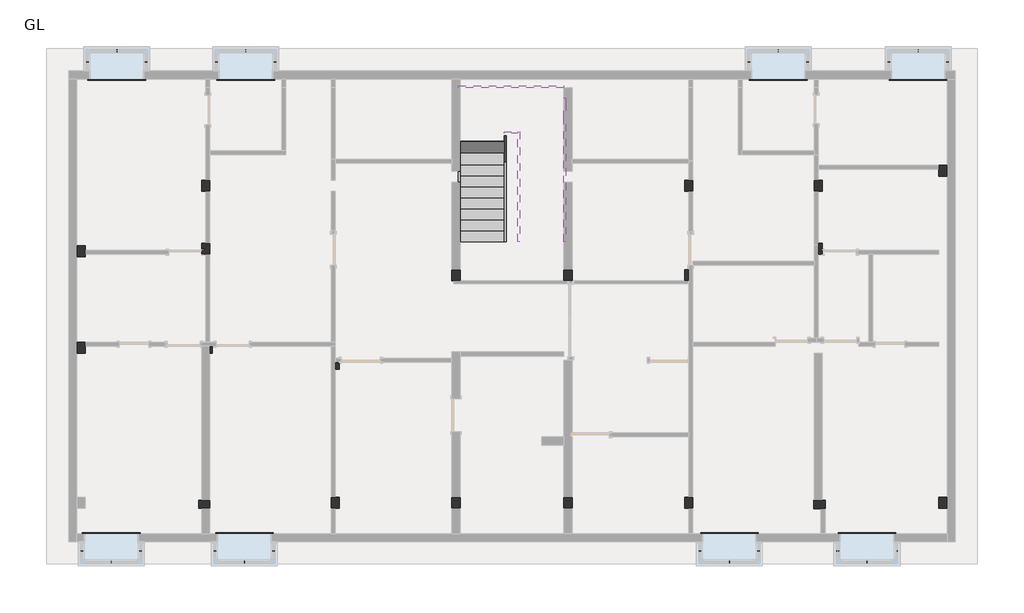
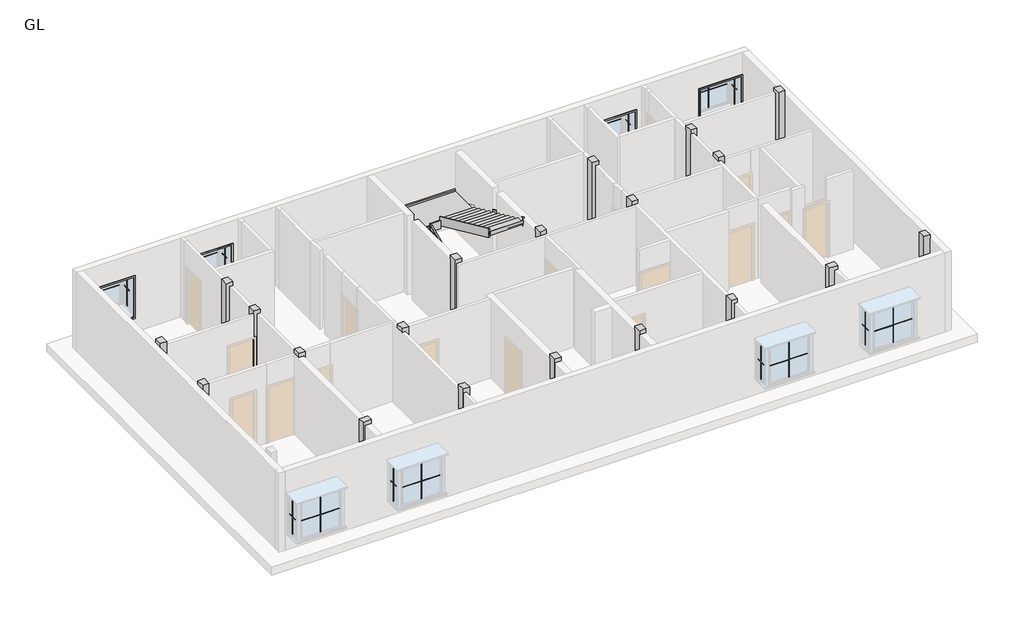
# One storey, part 3 of 3: 32 proxies, 20 columns, 6 members, 1 stair flight.
"""IFC4 building model written with IfcOpenShell, lengths in millimetres."""

from ifc_helpers import new_model, si_unit, frame, origin, place, context, project, spatial, polyline, outline, extrude, faceted_brep, transform, mapped, element, save
from components import m_muntin_pattern_2x2_m_muntin_pattern_2x2_c1fd4460, m_muntin_pattern_2x2_m_muntin_pattern_2x2_777b163a, m_trim_window_interior_flat_picture_frame_44e8afef, stair_flight_f8c5991c

model = new_model("IFC4")

# Units and contexts
model_context = context("Model", 3, world=origin())
ifc_project = project(units=[si_unit("LENGTHUNIT", "METRE", prefix="MILLI")], contexts=[model_context])

# Site, building, storey
site = spatial("IfcSite", under=ifc_project)
building = spatial("IfcBuilding", under=site)
storey = spatial("IfcBuildingStorey", under=building, Name="GL", Elevation=3200.4)

# Proxies
placement = place(None, origin())
m_muntin_pattern_2x2_m_muntin_pattern_2x2_shape = m_muntin_pattern_2x2_m_muntin_pattern_2x2_c1fd4460(model_context)
element("IfcBuildingElementProxy", 1, Name="M_Muntin Pattern_2x2 : M_Muntin Pattern_2x2", ObjectType="M_Muntin Pattern_2x2 : M_Muntin Pattern_2x2", at=placement, inside=storey, context=model_context, shape_type="MappedRepresentation", body=[
    mapped(m_muntin_pattern_2x2_m_muntin_pattern_2x2_shape, transform((-11500.7987957, -5499.9182661, 3921.05), x_axis=(-1.0, 0.0, 0.0), y_axis=(0.0, -1.0, 0.0), z_axis=(0.0, 0.0, 1.0))),
])
element("IfcBuildingElementProxy", 2, Name="M_Muntin Pattern_2x2 : M_Muntin Pattern_2x2", ObjectType="M_Muntin Pattern_2x2 : M_Muntin Pattern_2x2", at=placement, inside=storey, context=model_context, shape_type="MappedRepresentation", body=[
    mapped(m_muntin_pattern_2x2_m_muntin_pattern_2x2_shape, transform((-7819.250543, -5499.9182661, 3921.05), x_axis=(-1.0, 0.0, 0.0), y_axis=(0.0, -1.0, 0.0), z_axis=(0.0, 0.0, 1.0))),
])
element("IfcBuildingElementProxy", 3, Name="M_Muntin Pattern_2x2 : M_Muntin Pattern_2x2", ObjectType="M_Muntin Pattern_2x2 : M_Muntin Pattern_2x2", at=placement, inside=storey, context=model_context, shape_type="MappedRepresentation", body=[
    mapped(m_muntin_pattern_2x2_m_muntin_pattern_2x2_shape, transform((5599.7512082, -5499.9182661, 3921.05), x_axis=(-1.0, 0.0, 0.0), y_axis=(0.0, -1.0, 0.0), z_axis=(0.0, 0.0, 1.0))),
])
element("IfcBuildingElementProxy", 4, Name="M_Muntin Pattern_2x2 : M_Muntin Pattern_2x2", ObjectType="M_Muntin Pattern_2x2 : M_Muntin Pattern_2x2", at=placement, inside=storey, context=model_context, shape_type="MappedRepresentation", body=[
    mapped(m_muntin_pattern_2x2_m_muntin_pattern_2x2_shape, transform((9408.6146942, -5499.9182662, 3921.05), x_axis=(-1.0, 0.0, 0.0), y_axis=(0.0, -1.0, 0.0), z_axis=(0.0, 0.0, 1.0))),
])
element("IfcBuildingElementProxy", 5, Name="M_Muntin Pattern_2x2 : M_Muntin Pattern_2x2", ObjectType="M_Muntin Pattern_2x2 : M_Muntin Pattern_2x2", at=placement, inside=storey, context=model_context, shape_type="MappedRepresentation", body=[
    mapped(m_muntin_pattern_2x2_m_muntin_pattern_2x2_shape, transform((-11348.3987957, 8647.7317329, 3921.05), x_axis=(1.0, 0.0, 0.0), y_axis=(0.0, 1.0, 0.0), z_axis=(0.0, 0.0, 1.0))),
])
element("IfcBuildingElementProxy", 6, Name="M_Muntin Pattern_2x2 : M_Muntin Pattern_2x2", ObjectType="M_Muntin Pattern_2x2 : M_Muntin Pattern_2x2", at=placement, inside=storey, context=model_context, shape_type="MappedRepresentation", body=[
    mapped(m_muntin_pattern_2x2_m_muntin_pattern_2x2_shape, transform((-7779.6987993, 8647.7317329, 3921.05), x_axis=(1.0, 0.0, 0.0), y_axis=(0.0, 1.0, 0.0), z_axis=(0.0, 0.0, 1.0))),
])
element("IfcBuildingElementProxy", 7, Name="M_Muntin Pattern_2x2 : M_Muntin Pattern_2x2", ObjectType="M_Muntin Pattern_2x2 : M_Muntin Pattern_2x2", at=placement, inside=storey, context=model_context, shape_type="MappedRepresentation", body=[
    mapped(m_muntin_pattern_2x2_m_muntin_pattern_2x2_shape, transform((6952.301208, 8647.7317329, 3921.05), x_axis=(1.0, 0.0, 0.0), y_axis=(0.0, 1.0, 0.0), z_axis=(0.0, 0.0, 1.0))),
])
element("IfcBuildingElementProxy", 8, Name="M_Muntin Pattern_2x2 : M_Muntin Pattern_2x2", ObjectType="M_Muntin Pattern_2x2 : M_Muntin Pattern_2x2", at=placement, inside=storey, context=model_context, shape_type="MappedRepresentation", body=[
    mapped(m_muntin_pattern_2x2_m_muntin_pattern_2x2_shape, transform((10825.8012075, 8647.7317329, 3921.05), x_axis=(1.0, 0.0, 0.0), y_axis=(0.0, 1.0, 0.0), z_axis=(0.0, 0.0, 1.0))),
])
m_muntin_pattern_2x2_m_muntin_pattern_2x2_2_shape = m_muntin_pattern_2x2_m_muntin_pattern_2x2_777b163a(model_context)
element("IfcBuildingElementProxy", 9, Name="M_Muntin Pattern_2x2 : M_Muntin Pattern_2x2", ObjectType="M_Muntin Pattern_2x2 : M_Muntin Pattern_2x2", at=placement, inside=storey, context=model_context, shape_type="MappedRepresentation", body=[
    mapped(m_muntin_pattern_2x2_m_muntin_pattern_2x2_2_shape, transform((-10690.4737957, -5190.3932661, 3921.05), x_axis=(0.0, 1.0, 0.0), y_axis=(-1.0, 0.0, 0.0), z_axis=(0.0, 0.0, 1.0))),
])
element("IfcBuildingElementProxy", 10, Name="M_Muntin Pattern_2x2 : M_Muntin Pattern_2x2", ObjectType="M_Muntin Pattern_2x2 : M_Muntin Pattern_2x2", at=placement, inside=storey, context=model_context, shape_type="MappedRepresentation", body=[
    mapped(m_muntin_pattern_2x2_m_muntin_pattern_2x2_2_shape, transform((-12311.1237957, -5190.3932661, 3921.05), x_axis=(0.0, -1.0, 0.0), y_axis=(1.0, 0.0, 0.0), z_axis=(0.0, 0.0, 1.0))),
])
element("IfcBuildingElementProxy", 11, Name="M_Muntin Pattern_2x2 : M_Muntin Pattern_2x2", ObjectType="M_Muntin Pattern_2x2 : M_Muntin Pattern_2x2", at=placement, inside=storey, context=model_context, shape_type="MappedRepresentation", body=[
    mapped(m_muntin_pattern_2x2_m_muntin_pattern_2x2_2_shape, transform((-7008.925543, -5190.3932661, 3921.05), x_axis=(0.0, 1.0, 0.0), y_axis=(-1.0, 0.0, 0.0), z_axis=(0.0, 0.0, 1.0))),
])
element("IfcBuildingElementProxy", 12, Name="M_Muntin Pattern_2x2 : M_Muntin Pattern_2x2", ObjectType="M_Muntin Pattern_2x2 : M_Muntin Pattern_2x2", at=placement, inside=storey, context=model_context, shape_type="MappedRepresentation", body=[
    mapped(m_muntin_pattern_2x2_m_muntin_pattern_2x2_2_shape, transform((-8629.575543, -5190.3932661, 3921.05), x_axis=(0.0, -1.0, 0.0), y_axis=(1.0, 0.0, 0.0), z_axis=(0.0, 0.0, 1.0))),
])
element("IfcBuildingElementProxy", 13, Name="M_Muntin Pattern_2x2 : M_Muntin Pattern_2x2", ObjectType="M_Muntin Pattern_2x2 : M_Muntin Pattern_2x2", at=placement, inside=storey, context=model_context, shape_type="MappedRepresentation", body=[
    mapped(m_muntin_pattern_2x2_m_muntin_pattern_2x2_2_shape, transform((6410.0762082, -5190.3932661, 3921.05), x_axis=(0.0, 1.0, 0.0), y_axis=(-1.0, 0.0, 0.0), z_axis=(0.0, 0.0, 1.0))),
])
element("IfcBuildingElementProxy", 14, Name="M_Muntin Pattern_2x2 : M_Muntin Pattern_2x2", ObjectType="M_Muntin Pattern_2x2 : M_Muntin Pattern_2x2", at=placement, inside=storey, context=model_context, shape_type="MappedRepresentation", body=[
    mapped(m_muntin_pattern_2x2_m_muntin_pattern_2x2_2_shape, transform((4789.4262082, -5190.3932661, 3921.05), x_axis=(0.0, -1.0, 0.0), y_axis=(1.0, 0.0, 0.0), z_axis=(0.0, 0.0, 1.0))),
])
element("IfcBuildingElementProxy", 15, Name="M_Muntin Pattern_2x2 : M_Muntin Pattern_2x2", ObjectType="M_Muntin Pattern_2x2 : M_Muntin Pattern_2x2", at=placement, inside=storey, context=model_context, shape_type="MappedRepresentation", body=[
    mapped(m_muntin_pattern_2x2_m_muntin_pattern_2x2_2_shape, transform((10218.9396942, -5190.3932662, 3921.05), x_axis=(0.0, 1.0, 0.0), y_axis=(-1.0, 0.0, 0.0), z_axis=(0.0, 0.0, 1.0))),
])
element("IfcBuildingElementProxy", 16, Name="M_Muntin Pattern_2x2 : M_Muntin Pattern_2x2", ObjectType="M_Muntin Pattern_2x2 : M_Muntin Pattern_2x2", at=placement, inside=storey, context=model_context, shape_type="MappedRepresentation", body=[
    mapped(m_muntin_pattern_2x2_m_muntin_pattern_2x2_2_shape, transform((8598.2896942, -5190.3932661, 3921.05), x_axis=(0.0, -1.0, 0.0), y_axis=(1.0, 0.0, 0.0), z_axis=(0.0, 0.0, 1.0))),
])
element("IfcBuildingElementProxy", 17, Name="M_Muntin Pattern_2x2 : M_Muntin Pattern_2x2", ObjectType="M_Muntin Pattern_2x2 : M_Muntin Pattern_2x2", at=placement, inside=storey, context=model_context, shape_type="MappedRepresentation", body=[
    mapped(m_muntin_pattern_2x2_m_muntin_pattern_2x2_2_shape, transform((-12158.7237957, 8338.2067329, 3921.05), x_axis=(0.0, -1.0, 0.0), y_axis=(1.0, 0.0, 0.0), z_axis=(0.0, 0.0, 1.0))),
])
element("IfcBuildingElementProxy", 18, Name="M_Muntin Pattern_2x2 : M_Muntin Pattern_2x2", ObjectType="M_Muntin Pattern_2x2 : M_Muntin Pattern_2x2", at=placement, inside=storey, context=model_context, shape_type="MappedRepresentation", body=[
    mapped(m_muntin_pattern_2x2_m_muntin_pattern_2x2_2_shape, transform((-10538.0737957, 8338.2067329, 3921.05), x_axis=(0.0, 1.0, 0.0), y_axis=(-1.0, 0.0, 0.0), z_axis=(0.0, 0.0, 1.0))),
])
element("IfcBuildingElementProxy", 19, Name="M_Muntin Pattern_2x2 : M_Muntin Pattern_2x2", ObjectType="M_Muntin Pattern_2x2 : M_Muntin Pattern_2x2", at=placement, inside=storey, context=model_context, shape_type="MappedRepresentation", body=[
    mapped(m_muntin_pattern_2x2_m_muntin_pattern_2x2_2_shape, transform((-8590.0237993, 8338.2067329, 3921.05), x_axis=(0.0, -1.0, 0.0), y_axis=(1.0, 0.0, 0.0), z_axis=(0.0, 0.0, 1.0))),
])
element("IfcBuildingElementProxy", 20, Name="M_Muntin Pattern_2x2 : M_Muntin Pattern_2x2", ObjectType="M_Muntin Pattern_2x2 : M_Muntin Pattern_2x2", at=placement, inside=storey, context=model_context, shape_type="MappedRepresentation", body=[
    mapped(m_muntin_pattern_2x2_m_muntin_pattern_2x2_2_shape, transform((-6969.3737993, 8338.2067329, 3921.05), x_axis=(0.0, 1.0, 0.0), y_axis=(-1.0, 0.0, 0.0), z_axis=(0.0, 0.0, 1.0))),
])
element("IfcBuildingElementProxy", 21, Name="M_Muntin Pattern_2x2 : M_Muntin Pattern_2x2", ObjectType="M_Muntin Pattern_2x2 : M_Muntin Pattern_2x2", at=placement, inside=storey, context=model_context, shape_type="MappedRepresentation", body=[
    mapped(m_muntin_pattern_2x2_m_muntin_pattern_2x2_2_shape, transform((6141.976208, 8338.2067329, 3921.05), x_axis=(0.0, -1.0, 0.0), y_axis=(1.0, 0.0, 0.0), z_axis=(0.0, 0.0, 1.0))),
])
element("IfcBuildingElementProxy", 22, Name="M_Muntin Pattern_2x2 : M_Muntin Pattern_2x2", ObjectType="M_Muntin Pattern_2x2 : M_Muntin Pattern_2x2", at=placement, inside=storey, context=model_context, shape_type="MappedRepresentation", body=[
    mapped(m_muntin_pattern_2x2_m_muntin_pattern_2x2_2_shape, transform((7762.626208, 8338.2067329, 3921.05), x_axis=(0.0, 1.0, 0.0), y_axis=(-1.0, 0.0, 0.0), z_axis=(0.0, 0.0, 1.0))),
])
element("IfcBuildingElementProxy", 23, Name="M_Muntin Pattern_2x2 : M_Muntin Pattern_2x2", ObjectType="M_Muntin Pattern_2x2 : M_Muntin Pattern_2x2", at=placement, inside=storey, context=model_context, shape_type="MappedRepresentation", body=[
    mapped(m_muntin_pattern_2x2_m_muntin_pattern_2x2_2_shape, transform((10015.4762075, 8338.2067329, 3921.05), x_axis=(0.0, -1.0, 0.0), y_axis=(1.0, 0.0, 0.0), z_axis=(0.0, 0.0, 1.0))),
])
element("IfcBuildingElementProxy", 24, Name="M_Muntin Pattern_2x2 : M_Muntin Pattern_2x2", ObjectType="M_Muntin Pattern_2x2 : M_Muntin Pattern_2x2", at=placement, inside=storey, context=model_context, shape_type="MappedRepresentation", body=[
    mapped(m_muntin_pattern_2x2_m_muntin_pattern_2x2_2_shape, transform((11636.1262075, 8338.2067329, 3921.05), x_axis=(0.0, 1.0, 0.0), y_axis=(-1.0, 0.0, 0.0), z_axis=(0.0, 0.0, 1.0))),
])
m_trim_window_interior_flat_picture_frame_shape = m_trim_window_interior_flat_picture_frame_44e8afef(model_context)
element("IfcBuildingElementProxy", 25, Name="M_Trim-Window-Interior-Flat : Picture Frame", ObjectType="M_Trim-Window-Interior-Flat : Picture Frame", at=placement, inside=storey, context=model_context, shape_type="MappedRepresentation", body=[
    mapped(m_trim_window_interior_flat_picture_frame_shape, transform((-11500.7987957, -4712.5932661, 5351.2), x_axis=(-1.0, 0.0, 0.0), y_axis=(0.0, 0.0, 1.0), z_axis=(0.0, 1.0, 0.0))),
])
element("IfcBuildingElementProxy", 26, Name="M_Trim-Window-Interior-Flat : Picture Frame", ObjectType="M_Trim-Window-Interior-Flat : Picture Frame", at=placement, inside=storey, context=model_context, shape_type="MappedRepresentation", body=[
    mapped(m_trim_window_interior_flat_picture_frame_shape, transform((-7819.250543, -4712.5932661, 5351.2), x_axis=(-1.0, 0.0, 0.0), y_axis=(0.0, 0.0, 1.0), z_axis=(0.0, 1.0, 0.0))),
])
element("IfcBuildingElementProxy", 27, Name="M_Trim-Window-Interior-Flat : Picture Frame", ObjectType="M_Trim-Window-Interior-Flat : Picture Frame", at=placement, inside=storey, context=model_context, shape_type="MappedRepresentation", body=[
    mapped(m_trim_window_interior_flat_picture_frame_shape, transform((5599.7512082, -4712.5932661, 5351.2), x_axis=(-1.0, 0.0, 0.0), y_axis=(0.0, 0.0, 1.0), z_axis=(0.0, 1.0, 0.0))),
])
element("IfcBuildingElementProxy", 28, Name="M_Trim-Window-Interior-Flat : Picture Frame", ObjectType="M_Trim-Window-Interior-Flat : Picture Frame", at=placement, inside=storey, context=model_context, shape_type="MappedRepresentation", body=[
    mapped(m_trim_window_interior_flat_picture_frame_shape, transform((9408.6146942, -4712.5932661, 5351.2), x_axis=(-1.0, 0.0, 0.0), y_axis=(0.0, 0.0, 1.0), z_axis=(0.0, 1.0, 0.0))),
])
element("IfcBuildingElementProxy", 29, Name="M_Trim-Window-Interior-Flat : Picture Frame", ObjectType="M_Trim-Window-Interior-Flat : Picture Frame", at=placement, inside=storey, context=model_context, shape_type="MappedRepresentation", body=[
    mapped(m_trim_window_interior_flat_picture_frame_shape, transform((-11348.3987957, 7860.4067329, 5351.2), x_axis=(1.0, 0.0, 0.0), y_axis=(0.0, 0.0, 1.0), z_axis=(0.0, -1.0, 0.0))),
])
element("IfcBuildingElementProxy", 30, Name="M_Trim-Window-Interior-Flat : Picture Frame", ObjectType="M_Trim-Window-Interior-Flat : Picture Frame", at=placement, inside=storey, context=model_context, shape_type="MappedRepresentation", body=[
    mapped(m_trim_window_interior_flat_picture_frame_shape, transform((-7779.6987993, 7860.4067329, 5351.2), x_axis=(1.0, 0.0, 0.0), y_axis=(0.0, 0.0, 1.0), z_axis=(0.0, -1.0, 0.0))),
])
element("IfcBuildingElementProxy", 31, Name="M_Trim-Window-Interior-Flat : Picture Frame", ObjectType="M_Trim-Window-Interior-Flat : Picture Frame", at=placement, inside=storey, context=model_context, shape_type="MappedRepresentation", body=[
    mapped(m_trim_window_interior_flat_picture_frame_shape, transform((6952.301208, 7860.4067329, 5351.2), x_axis=(1.0, 0.0, 0.0), y_axis=(0.0, 0.0, 1.0), z_axis=(0.0, -1.0, 0.0))),
])
element("IfcBuildingElementProxy", 32, Name="M_Trim-Window-Interior-Flat : Picture Frame", ObjectType="M_Trim-Window-Interior-Flat : Picture Frame", at=placement, inside=storey, context=model_context, shape_type="MappedRepresentation", body=[
    mapped(m_trim_window_interior_flat_picture_frame_shape, transform((10825.8012075, 7860.4067329, 5351.2), x_axis=(1.0, 0.0, 0.0), y_axis=(0.0, 0.0, 1.0), z_axis=(0.0, -1.0, 0.0))),
])

# Columns
element("IfcColumn", 33, ObjectType="Rectangular Column : 1'X 9\"", at=placement, inside=storey, context=model_context, shape_type="SweptSolid", body=[
    extrude(outline(polyline([(-12224.6987957, 583.3067334), (-12224.6987957, 278.5067334), (-12453.2987957, 278.5067334), (-12453.2987957, 583.3067334), (-12224.6987957, 583.3067334)])), frame((0.0, 0.0, 3200.4), z_axis=(0.0, 0.0, 1.0), x_axis=(1.0, 0.0, 0.0)), (0.0, 0.0, 1.0), 3200.4),
])
element("IfcColumn", 34, ObjectType="Rectangular Column : 1'X 9\"", at=placement, inside=storey, context=model_context, shape_type="SweptSolid", body=[
    extrude(outline(polyline([(-12224.6987957, 3256.6567332), (-12224.6987957, 2951.8567332), (-12453.2987957, 2951.8567332), (-12453.2987957, 3256.6567332), (-12224.6987957, 3256.6567332)])), frame((0.0, 0.0, 3200.4), z_axis=(0.0, 0.0, 1.0), x_axis=(1.0, 0.0, 0.0)), (0.0, 0.0, 1.0), 3200.4),
])
element("IfcColumn", 35, ObjectType="Rectangular Column : 1'X 9\"", at=placement, inside=storey, context=model_context, shape_type="Brep", body=[
    faceted_brep([(-8770.2987992, 5066.406733, 3200.4), (-8770.2987992, 4761.606733, 3200.4), (-8884.5987992, 4761.606733, 3200.4), (-8998.8987992, 4761.606733, 3200.4), (-8998.8987992, 5066.406733, 3200.4), (-8884.5987992, 5066.406733, 3200.4), (-8770.2987992, 5066.406733, 6400.8), (-8770.2987992, 4761.606733, 6400.8), (-8770.2987992, 4761.606733, 6248.4), (-8770.2987992, 5066.406733, 6248.4), (-8998.8987992, 4761.606733, 6400.8), (-8998.8987992, 5066.406733, 6400.8)], [[[0, 1, 2, 3, 4, 5]], [[6, 7, 8, 1, 0, 9]], [[7, 10, 3, 2, 1, 8]], [[10, 11, 4, 3]], [[11, 6, 9, 0, 5, 4]], [[6, 11, 10, 7]]]),
])
element("IfcColumn", 36, ObjectType="Rectangular Column : 1'X 9\"", at=placement, inside=storey, context=model_context, shape_type="Brep", body=[
    faceted_brep([(-8770.2987992, 3326.5067332, 3200.4), (-8770.2987992, 3021.7067332, 3200.4), (-8884.598796, 3021.7067332, 3200.4), (-8998.8987992, 3021.7067332, 3200.4), (-8998.8987992, 3326.5067332, 3200.4), (-8884.5987992, 3326.5067332, 3200.4), (-8770.2987992, 3326.5067332, 6400.8), (-8770.2987992, 3021.7067332, 6400.8), (-8770.2987992, 3326.5067332, 6248.4), (-8998.8987992, 3021.7067332, 6400.8), (-8998.8987992, 3326.5067332, 6400.8)], [[[0, 1, 2, 3, 4, 5]], [[6, 7, 1, 0, 8]], [[7, 9, 3, 2, 1]], [[9, 10, 4, 3]], [[10, 6, 8, 0, 5, 4]], [[6, 10, 9, 7]]]),
])
element("IfcColumn", 37, ObjectType="Rectangular Column : 1'X 9\"", at=placement, inside=storey, context=model_context, shape_type="Brep", body=[
    faceted_brep([(-8713.148796, 278.5067334, 3200.4), (-8771.750543, 278.5067334, 3200.4), (-8771.750543, 469.0067334, 3200.4), (-8713.148796, 469.0067334, 3200.4), (-8713.148796, 583.3067334, 6400.8), (-8713.148796, 278.5067334, 6400.8), (-8713.148796, 469.0067334, 6248.4), (-8713.148796, 583.3067334, 6248.4), (-8941.748796, 278.5067334, 6400.8), (-8941.748796, 278.5067334, 6248.4), (-8771.750543, 278.5067334, 6248.4), (-8941.748796, 583.3067334, 6400.8), (-8941.748796, 583.3067334, 6248.4), (-8941.748796, 469.0067334, 6248.4), (-8771.750543, 469.0067334, 6248.4)], [[[0, 1, 2, 3]], [[4, 5, 0, 3, 6, 7]], [[0, 5, 8, 9, 10, 1]], [[8, 11, 12, 13, 9]], [[11, 4, 7, 12]], [[5, 4, 11, 8]], [[10, 14, 2, 1]], [[14, 10, 9, 13]], [[14, 6, 3, 2]], [[6, 14, 13, 12, 7]]]),
])
element("IfcColumn", 38, ObjectType="Rectangular Column : 1'X 9\"", at=placement, inside=storey, context=model_context, shape_type="Brep", body=[
    faceted_brep([(-9076.550543, -3785.4932196, 3200.4), (-9000.350543, -3785.4932196, 3200.4), (-8771.750543, -3785.4932196, 3200.4), (-8771.750543, -4014.0932196, 3200.4), (-9000.350543, -4014.0932196, 3200.4), (-9076.550543, -4014.0932196, 3200.4), (-9076.550543, -3785.4932196, 6400.8), (-8771.750543, -3785.4932196, 6400.8), (-8771.750543, -3785.4932196, 6248.4), (-8771.750543, -4014.0932196, 6400.8), (-8771.750543, -4014.0932196, 6248.4), (-9076.550543, -4014.0932196, 6400.8)], [[[0, 1, 2, 3, 4, 5]], [[6, 7, 8, 2, 1, 0]], [[7, 9, 10, 3, 2, 8]], [[9, 11, 5, 4, 3, 10]], [[11, 6, 0, 5]], [[6, 11, 9, 7]]]),
])
element("IfcColumn", 39, ObjectType="Rectangular Column : 1'X 9\"", at=placement, inside=storey, context=model_context, shape_type="Brep", body=[
    faceted_brep([(-5417.4987963, -4014.0932193, 3200.4), (-5417.4987963, -3709.2932193, 3200.4), (-5303.1987995, -3709.2932193, 3200.4), (-5188.8987963, -3709.2932193, 3200.4), (-5188.8987963, -4014.0932193, 3200.4), (-5303.1987963, -4014.0932193, 3200.4), (-5417.4987963, -4014.0932193, 6400.8), (-5417.4987963, -3709.2932193, 6400.8), (-5417.4987963, -4014.0932193, 6248.4), (-5188.8987963, -3709.2932193, 6400.8), (-5188.8987963, -4014.0932193, 6400.8)], [[[0, 1, 2, 3, 4, 5]], [[6, 7, 1, 0, 8]], [[7, 9, 3, 2, 1]], [[9, 10, 4, 3]], [[10, 6, 8, 0, 5, 4]], [[6, 10, 9, 7]]]),
])
element("IfcColumn", 40, ObjectType="Rectangular Column : 1'X 9\"", at=placement, inside=storey, context=model_context, shape_type="Brep", body=[
    faceted_brep([(-2077.3987998, -4014.0932663, 3200.4), (-2077.3987998, -3709.2932663, 3200.4), (-1848.7987998, -3709.2932663, 3200.4), (-1848.7987998, -4014.0932663, 3200.4), (-2077.3987998, -4014.0932663, 6400.8), (-2077.3987998, -3709.2932663, 6400.8), (-2077.3987998, -3709.2932663, 6248.4), (-2077.3987998, -4014.0932663, 6248.4), (-1848.7987998, -3709.2932663, 6400.8), (-1848.7987998, -3709.2932663, 6248.4), (-1848.7987998, -4014.0932663, 6400.8), (-1848.7987998, -4014.0932663, 6248.4)], [[[0, 1, 2, 3]], [[4, 5, 6, 1, 0, 7]], [[5, 8, 9, 2, 1, 6]], [[8, 10, 11, 3, 2, 9]], [[10, 4, 7, 0, 3, 11]], [[4, 10, 8, 5]]]),
])
element("IfcColumn", 41, ObjectType="Rectangular Column : 1'X 9\"", at=placement, inside=storey, context=model_context, shape_type="Brep", body=[
    faceted_brep([(1021.4012085, -4014.0932193, 3200.4), (1021.4012085, -3709.2932193, 3200.4), (1250.0012085, -3709.2932193, 3200.4), (1250.0012085, -4014.0932193, 3200.4), (1021.4012085, -4014.0932193, 6400.8), (1021.4012085, -3709.2932193, 6400.8), (1021.4012085, -3709.2932193, 6248.4), (1021.4012085, -4014.0932193, 6248.4), (1250.0012085, -3709.2932193, 6400.8), (1250.0012085, -3709.2932193, 6248.4), (1250.0012085, -4014.0932193, 6400.8), (1250.0012085, -4014.0932193, 6248.4)], [[[0, 1, 2, 3]], [[4, 5, 6, 1, 0, 7]], [[5, 8, 9, 2, 1, 6]], [[8, 10, 11, 3, 2, 9]], [[10, 4, 7, 0, 3, 11]], [[4, 10, 8, 5]]]),
])
element("IfcColumn", 42, ObjectType="Rectangular Column : 1'X 9\"", at=placement, inside=storey, context=model_context, shape_type="Brep", body=[
    faceted_brep([(4361.5012082, -4014.0932193, 3200.4), (4361.5012082, -3709.2932193, 3200.4), (4475.8012082, -3709.2932193, 3200.4), (4590.1012082, -3709.2932193, 3200.4), (4590.1012082, -4014.0932193, 3200.4), (4475.8012082, -4014.0932193, 3200.4), (4361.5012082, -4014.0932193, 6400.8), (4361.5012082, -3709.2932193, 6400.8), (4590.1012082, -3709.2932193, 6400.8), (4590.1012082, -3709.2932193, 6248.4), (4590.1012082, -4014.0932193, 6400.8), (4590.1012082, -4014.0932193, 6248.4)], [[[0, 1, 2, 3, 4, 5]], [[6, 7, 1, 0]], [[7, 8, 9, 3, 2, 1]], [[8, 10, 11, 4, 3, 9]], [[10, 6, 0, 5, 4, 11]], [[6, 10, 8, 7]]]),
])
element("IfcColumn", 43, ObjectType="Rectangular Column : 1'X 9\"", at=placement, inside=storey, context=model_context, shape_type="Brep", body=[
    faceted_brep([(8246.5646942, -4015.9914801, 3200.4), (8132.2646942, -4015.9914801, 3200.4), (7941.7646942, -4015.9914801, 3200.4), (7941.7646942, -3787.3914801, 3200.4), (8246.5646942, -3787.3914801, 3200.4), (8246.5646942, -4015.9914801, 6400.8), (7941.7646942, -4015.9914801, 6400.8), (8246.5646942, -4015.9914801, 6248.4), (7941.7646942, -3787.3914801, 6400.8), (8246.5646942, -3787.3914801, 6400.8)], [[[0, 1, 2, 3, 4]], [[5, 6, 2, 1, 0, 7]], [[6, 8, 3, 2]], [[8, 9, 4, 3]], [[9, 5, 7, 0, 4]], [[5, 9, 8, 6]]]),
])
element("IfcColumn", 44, ObjectType="Rectangular Column : 1'X 9\"", at=placement, inside=storey, context=model_context, shape_type="SweptSolid", body=[
    extrude(outline(polyline([(11625.9012075, -3709.2932671), (11625.9012075, -4014.0932671), (11397.3012075, -4014.0932671), (11397.3012075, -3709.2932671), (11625.9012075, -3709.2932671)])), frame((0.0, 0.0, 3200.4), z_axis=(0.0, 0.0, 1.0), x_axis=(1.0, 0.0, 0.0)), (0.0, 0.0, 1.0), 3200.4),
])
element("IfcColumn", 45, ObjectType="Rectangular Column : 1'X 9\"", at=placement, inside=storey, context=model_context, shape_type="Brep", body=[
    faceted_brep([(11625.9012075, 5479.1567329, 3200.4), (11625.9012075, 5174.3567329, 3200.4), (11397.3012075, 5174.3567329, 3200.4), (11397.3012075, 5364.8567329, 3200.4), (11397.3012075, 5479.1567329, 3200.4), (11625.9012075, 5479.1567329, 6400.8), (11625.9012075, 5174.3567329, 6400.8), (11397.3012075, 5174.3567329, 6400.8), (11397.3012075, 5479.1567329, 6400.8), (11397.3012075, 5479.1567329, 6248.4)], [[[0, 1, 2, 3, 4]], [[5, 6, 1, 0]], [[6, 7, 2, 1]], [[7, 8, 9, 4, 3, 2]], [[8, 5, 0, 4, 9]], [[5, 8, 7, 6]]]),
])
element("IfcColumn", 46, ObjectType="Rectangular Column : 1'X 9\"", at=placement, inside=storey, context=model_context, shape_type="Brep", body=[
    faceted_brep([(8172.5040565, 5065.4824989, 3200.4), (8172.5040565, 4760.6824989, 3200.4), (8057.2012047, 4760.6824989, 3200.4), (7943.9040565, 4760.6824989, 3200.4), (7943.9040565, 5065.4824989, 3200.4), (8058.2040565, 5065.4824989, 3200.4), (8172.5040565, 5065.4824989, 6400.8), (8172.5040565, 4760.6824989, 6400.8), (7943.9040565, 4760.6824989, 6400.8), (7943.9040565, 5065.4824989, 6400.8), (7943.9040565, 5065.4824989, 6248.4)], [[[0, 1, 2, 3, 4, 5]], [[6, 7, 1, 0]], [[7, 8, 3, 2, 1]], [[8, 9, 10, 4, 3]], [[9, 6, 0, 5, 4, 10]], [[6, 9, 8, 7]]]),
])
element("IfcColumn", 47, ObjectType="Rectangular Column : 1'X 9\"", at=placement, inside=storey, context=model_context, shape_type="Brep", body=[
    faceted_brep([(8171.5012047, 3326.5067332, 3200.4), (8171.5012047, 3021.7067332, 3200.4), (8057.2012079, 3021.7067332, 3200.4), (8057.2012079, 3270.1432417, 3200.4), (8057.2012047, 3326.5067332, 3200.4), (8171.5012047, 3326.5067332, 6400.8), (8171.5012047, 3021.7067332, 6400.8), (7942.9012047, 3021.7067332, 6400.8), (7942.9012047, 3021.7067332, 6248.4), (8057.2012079, 3021.7067332, 6248.4), (7942.9012047, 3326.5067332, 6400.8), (7942.9012047, 3326.5067332, 6248.4), (7942.9012047, 3270.1432417, 6248.4), (8057.2012047, 3326.5067332, 6248.4), (8057.2012047, 3270.1432417, 6248.4)], [[[0, 1, 2, 3, 4]], [[1, 0, 5, 6]], [[1, 6, 7, 8, 9, 2]], [[7, 10, 11, 12, 8]], [[5, 0, 4, 13, 11, 10]], [[6, 5, 10, 7]], [[14, 13, 4, 3]], [[13, 14, 12, 11]], [[9, 14, 3, 2]], [[14, 9, 8, 12]]]),
])
element("IfcColumn", 48, ObjectType="Rectangular Column : 1'X 9\"", at=placement, inside=storey, context=model_context, shape_type="SweptSolid", body=[
    extrude(outline(polyline([(6400.8, 4590.1012082), (6400.8, 4361.5012082), (3200.4, 4361.5012082), (3200.4, 4475.8012082), (6248.4, 4475.8012082), (6248.4, 4590.1012082), (6400.8, 4590.1012082)])), frame((0.0, 2285.1067742, 0.0), z_axis=(0.0, 1.0, 0.0), x_axis=(0.0, 0.0, 1.0)), (0.0, 0.0, 1.0), 304.8),
])
element("IfcColumn", 49, ObjectType="Rectangular Column : 1'X 9\"", at=placement, inside=storey, context=model_context, shape_type="Brep", body=[
    faceted_brep([(4590.1012082, 5066.40678, 3200.4), (4590.1012082, 4761.60678, 3200.4), (4361.5012082, 4761.60678, 3200.4), (4361.5012082, 5066.40678, 3200.4), (4475.8012082, 5066.40678, 3200.4), (4590.1012082, 5066.40678, 6400.8), (4590.1012082, 4761.60678, 6400.8), (4590.1012082, 5066.40678, 6248.4), (4361.5012082, 4761.60678, 6400.8), (4361.5012082, 5066.40678, 6400.8)], [[[0, 1, 2, 3, 4]], [[5, 6, 1, 0, 7]], [[6, 8, 2, 1]], [[8, 9, 3, 2]], [[9, 5, 7, 0, 4, 3]], [[5, 9, 8, 6]]]),
])
element("IfcColumn", 50, ObjectType="Rectangular Column : 1'X 9\"", at=placement, inside=storey, context=model_context, shape_type="Brep", body=[
    faceted_brep([(1253.2582462, 2589.9067742, 3200.4), (1253.2582462, 2285.1067742, 3200.4), (1024.6582462, 2285.1067742, 3200.4), (1024.6582462, 2589.9067742, 3200.4), (1250.0012085, 2589.9067742, 3200.4), (1253.2582462, 2589.9067742, 6400.8), (1253.2582462, 2285.1067742, 6400.8), (1024.6582462, 2285.1067742, 6400.8), (1024.6582462, 2589.9067742, 6400.8)], [[[0, 1, 2, 3, 4]], [[5, 6, 1, 0]], [[6, 7, 2, 1]], [[7, 8, 3, 2]], [[8, 5, 0, 4, 3]], [[5, 8, 7, 6]]]),
])
element("IfcColumn", 51, ObjectType="Rectangular Column : 1'X 9\"", at=placement, inside=storey, context=model_context, shape_type="Brep", body=[
    faceted_brep([(-1845.5417538, 2589.906774, 3200.4), (-1845.5417538, 2285.106774, 3200.4), (-2020.2487998, 2285.106774, 3200.4), (-2074.1417538, 2285.106774, 3200.4), (-2074.1417538, 2589.906774, 3200.4), (-1845.5417538, 2589.906774, 6400.8), (-1845.5417538, 2285.106774, 6400.8), (-1845.5417538, 2589.906774, 6248.4), (-2074.1417538, 2285.106774, 6400.8), (-2074.1417538, 2589.906774, 6400.8), (-2074.1417538, 2589.906774, 6248.4)], [[[0, 1, 2, 3, 4]], [[5, 6, 1, 0, 7]], [[6, 8, 3, 2, 1]], [[8, 9, 10, 4, 3]], [[9, 5, 7, 0, 4, 10]], [[5, 9, 8, 6]]]),
])
element("IfcColumn", 52, ObjectType="Rectangular Column : 1'X 9\"", at=placement, inside=storey, context=model_context, shape_type="Brep", body=[
    faceted_brep([(-5188.8987995, 33.8078621, 3200.4), (-5188.8987995, -156.6921379, 3200.4), (-5303.1987995, -156.6921379, 3200.4), (-5303.1987995, 33.8078621, 3200.4), (-5188.8987995, 148.1078621, 6400.8), (-5188.8987995, -156.6921379, 6400.8), (-5188.8987995, 33.8078621, 6248.4), (-5188.8987995, 148.1078621, 6248.4), (-5417.4987995, -156.6921379, 6400.8), (-5417.4987995, -156.6921379, 6248.4), (-5303.1987995, -156.6921379, 6248.4), (-5417.4987995, 148.1078621, 6400.8), (-5417.4987995, 148.1078621, 6248.4), (-5303.1987995, 148.1078621, 6248.4), (-5303.1987995, 33.8078621, 6248.4)], [[[0, 1, 2, 3]], [[4, 5, 1, 0, 6, 7]], [[1, 5, 8, 9, 10, 2]], [[8, 11, 12, 9]], [[11, 4, 7, 13, 12]], [[5, 4, 11, 8]], [[14, 6, 0, 3]], [[6, 14, 13, 7]], [[10, 14, 3, 2]], [[14, 10, 9, 12, 13]]]),
])

# Members
element("IfcMember", 53, ObjectType="Stringer - 2\" Width", at=placement, inside=storey, context=model_context, shape_type="SweptSolid", body=[
    extrude(outline(polyline([(3364.6067329, 3200.4), (3364.6067329, 3400.2262721), (6445.4289342, 4800.6), (7182.0114168, 4800.6), (3661.5714168, 3200.4), (3364.6067329, 3200.4)])), frame((-1896.3417538, 0.0, 0.0), z_axis=(1.0, 0.0, 0.0), x_axis=(0.0, 1.0, 0.0)), (0.0, 0.0, 1.0), 50.8),
])
element("IfcMember", 54, ObjectType="Stringer - 2\" Width", at=placement, inside=storey, context=model_context, shape_type="SweptSolid", body=[
    extrude(outline(polyline([(-1896.3417538, 7631.8067329), (-1896.3417538, 7682.6067329), (1021.4012085, 7682.6067329), (1021.4012085, 7631.8067329), (-1896.3417538, 7631.8067329)])), frame((0.0, 0.0, 4495.8), z_axis=(0.0, 0.0, 1.0), x_axis=(1.0, 0.0, 0.0)), (0.0, 0.0, 1.0), 304.8),
])
element("IfcMember", 55, ObjectType="Stringer - 2\" Width", at=placement, inside=storey, context=model_context, shape_type="SweptSolid", body=[
    extrude(outline(polyline([(6618.562049, 4495.8), (3364.6067329, 5974.8705982), (3364.6067329, 6309.6808176), (7355.1445316, 4495.8), (6618.562049, 4495.8)])), frame((1021.4012085, 0.0, 0.0), z_axis=(1.0, 0.0, 0.0), x_axis=(0.0, 1.0, 0.0)), (0.0, 0.0, 1.0), 50.8),
])
element("IfcMember", 56, ObjectType="Stringer - 2\" Width", at=placement, inside=storey, context=model_context, shape_type="SweptSolid", body=[
    extrude(outline(polyline([(3364.6067329, 3200.4), (3364.6067329, 3400.2262721), (6361.8067329, 4762.5899085), (6361.8067329, 4427.7796892), (3661.5714168, 3200.4), (3364.6067329, 3200.4)])), frame((-629.5987998, 0.0, 0.0), z_axis=(1.0, 0.0, 0.0), x_axis=(0.0, 1.0, 0.0)), (0.0, 0.0, 1.0), 50.8),
])
element("IfcMember", 57, ObjectType="Stringer - 2\" Width", at=placement, inside=storey, context=model_context, shape_type="SweptSolid", body=[
    extrude(outline(polyline([(-629.5987998, 6361.8067329), (-629.5987998, 6412.6067329), (-248.5987915, 6412.6067329), (-248.5987915, 6361.8067329), (-629.5987998, 6361.8067329)])), frame((0.0, 0.0, 4495.8), z_axis=(0.0, 0.0, 1.0), x_axis=(1.0, 0.0, 0.0)), (0.0, 0.0, 1.0), 304.8),
])
element("IfcMember", 58, ObjectType="Stringer - 2\" Width", at=placement, inside=storey, context=model_context, shape_type="SweptSolid", body=[
    extrude(outline(polyline([(6412.6067329, 4924.2262721), (6412.6067329, 4589.4160528), (3364.6067329, 5974.8705982), (3364.6067329, 6309.6808176), (6412.6067329, 4924.2262721)])), frame((-248.5987915, 0.0, 0.0), z_axis=(1.0, 0.0, 0.0), x_axis=(0.0, 1.0, 0.0)), (0.0, 0.0, 1.0), 50.8),
])

# Stair flight
stair_flight_shape = stair_flight_f8c5991c(model_context)
element("IfcStairFlight", 59, ObjectType="2\" Tread 1\" Nosing 1/4\" Riser", at=placement, inside=storey, context=model_context, shape_type="MappedRepresentation", body=[
    mapped(stair_flight_shape, transform((0.0, 0.0, 0.0), x_axis=(1.0, 0.0, 0.0), y_axis=(0.0, 1.0, 0.0), z_axis=(0.0, 0.0, 1.0))),
])

save(model, "model.ifc")

# Revit data of these elements
# Type "M_Muntin Pattern_2x2 : M_Muntin Pattern_2x2"
#   Width [instance default] = 3' - 11.24409"
#   Thickness = 0' - 0 1/2"
#   Height [instance default] = 3' - 11.24409"
#   Distance = 0' - 0 3/4"
#   Interior Material [instance default] = none
#   Exterior Material [instance default] = none
#   Default Elevation = 0
# Type "M_Trim-Window-Interior-Flat : Picture Frame"
#   Trim Thickness_Picture Frame = 0' - 1.1811"
#   Trim Width = 0' - 2.3622"
#   Trim Thickness_with Sill = 0' - 0.7874"
#   Sill Thickness = 0' - 1.1811"
#   Opening Width [instance default] = 1' - 11.62205"
#   Opening Height [instance default] = 2' - 11.43307"
#   Default Elevation = 3' - 11.24409"
#   Sill = no
#   Picture Frame = yes
#   Trim Material [instance default] = none
# Type "Rectangular Column : 1'X 9\""
#   Assembly Code = "B1010200"
#   Depth = 1' - 0"
#   Offset Base = 0' - 0"
#   Offset Top = 0' - 0"
#   Width = 0' - 9"
#   Material = none
# Elements 1, 2, 3, 4, 5, 6, 7, 8 (IfcBuildingElementProxy, "M_Muntin Pattern_2x2 : M_Muntin Pattern_2x2")
#   Width = 4' - 5.55512"
#   Height = 4' - 5.55512"
#   Interior Material = Wood - Stained
#   Exterior Material = Clad - White
#   Phase Created = New Construction
#   Materials on its faces: "Clad - White", "Wood - Stained"
# Elements 9, 10, 11, 12, 13, 14, 15, 16, 17, 18, 19, 20, 21, 22, 23, 24 (IfcBuildingElementProxy, "M_Muntin Pattern_2x2 : M_Muntin Pattern_2x2")
#   Width = 1' - 2.12205"
#   Height = 4' - 5.55512"
#   Interior Material = Wood - Stained
#   Exterior Material = Clad - White
#   Phase Created = New Construction
#   Materials on its faces: "Clad - White", "Wood - Stained"
# Elements 25, 26, 27, 28, 29, 30, 31, 32 (IfcBuildingElementProxy, "M_Trim-Window-Interior-Flat : Picture Frame")
#   Opening Width = 4' - 11.05512"
#   Opening Height = 5' - 1.05512"
#   Trim Material = Wood - Stained
#   Phase Created = New Construction
#   Materials on its faces: "Wood - Stained"
# Elements 33, 34, 35, 36, 37, 38, 39, 40, 41, 42, 43, 44, 45, 46, 47, 48, 49, 50, 51, 52 (IfcColumn, "Rectangular Column : 1'X 9\"")
#   Phase Created = New Construction
#   Materials on its faces: "Default Wall"
# Elements 53, 54, 55, 56, 57, 58 (IfcMember, "Stringer - 2\" Width")
#   Phase Created = New Construction
# Element 59 (IfcStairFlight, "2\" Tread 1\" Nosing 1/4\" Riser")
#   Phase Created = New Construction
# Materials
#   "Clad - White": class "Wood", colour RGB 242 242 238, transparency 0, Cost = 0
#   "Wood - Stained": class "Wood", colour RGB 224 178 126, transparency 0, Cost = 0
#   "Default Wall": colour RGB 128 128 128, transparency 0, Cost = 0
